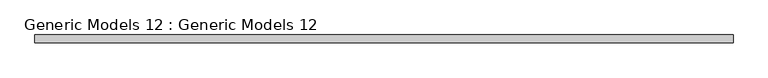
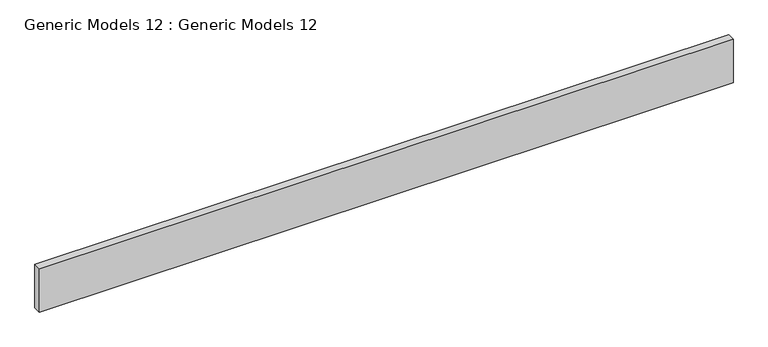
"""IFC4 building model written with IfcOpenShell, lengths in millimetres: proxy geometry, Generic Models 12 : Generic Models 12."""

from ifc_helpers import new_model, si_unit, frame, origin, place, context, project, spatial, polyline, outline, extrude, source, transform, mapped, element, save


def generic_models_12_generic_models_12_e4f72901(model_context):
    return source(origin(), model_context, "Body", "SweptSolid", [
        extrude(outline(polyline([(5870.7423568, -13324.1073314), (1273.3423568, -13324.1073314), (1273.3423568, -13273.3073314), (5870.7423568, -13273.3073314), (5870.7423568, -13324.1073314)])), frame((0.0, 0.0, 6400.8), z_axis=(0.0, 0.0, 1.0), x_axis=(1.0, 0.0, 0.0)), (0.0, 0.0, 1.0), 304.8),
    ])


if __name__ == "__main__":
    model = new_model("IFC4")
    model_context = context("Model", 3, world=origin())
    ifc_project = project(units=[si_unit("LENGTHUNIT", "METRE", prefix="MILLI")], contexts=[model_context])
    site = spatial("IfcSite", under=ifc_project)
    building = spatial("IfcBuilding", under=site)
    placement = place(None, origin())
    generic_models_12_generic_models_12_shape = generic_models_12_generic_models_12_e4f72901(model_context)
    element("IfcBuildingElementProxy", 1, Name="Generic Models 12 : Generic Models 12", ObjectType="Generic Models 12 : Generic Models 12", at=placement, inside=building, context=model_context, shape_type="MappedRepresentation", body=[
        mapped(generic_models_12_generic_models_12_shape, transform((0.0, 0.0, 0.0), x_axis=(1.0, 0.0, 0.0), y_axis=(0.0, 1.0, 0.0), z_axis=(0.0, 0.0, 1.0))),
    ])
    save(model, "model.ifc")

# Revit data of these elements
# Element 1 (IfcBuildingElementProxy, "Generic Models 12 : Generic Models 12")
#   Materials on its faces: "Clad - White"
# Materials
#   "Clad - White": class "Wood", colour RGB 242 242 238, transparency 0, Cost = 0
